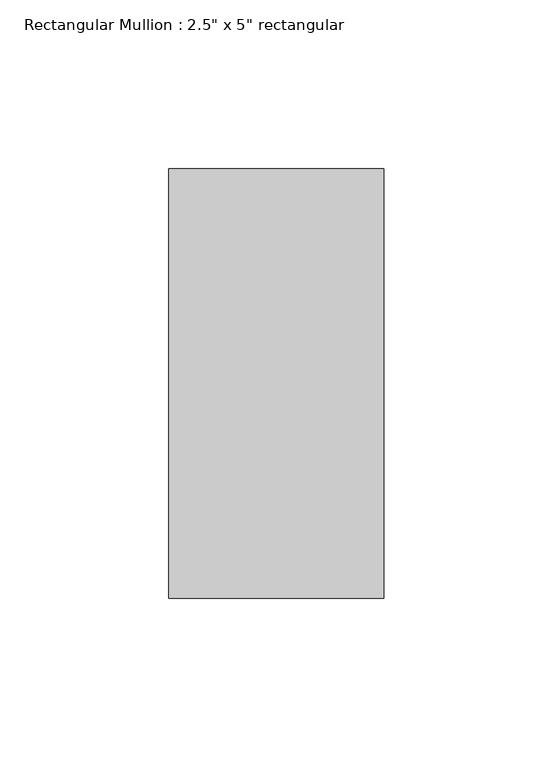
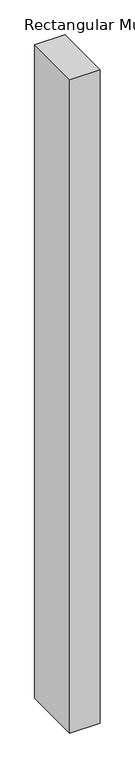
"""IFC4 building model written with IfcOpenShell, lengths in millimetres: member geometry."""

from ifc_helpers import new_model, si_unit, frame, origin, place, context, project, spatial, polyline, outline, extrude, source, transform, mapped, element, save


def member_b02ddeff(model_context):
    return source(origin(), model_context, "Body", "SweptSolid", [
        extrude(outline(polyline([(0.0, 63.5), (0.0, -63.5), (-63.5, -63.5), (-63.5, 63.5), (0.0, 63.5)])), frame((0.0, 0.0, -1446.9422272), z_axis=(0.0, 0.0, 1.0), x_axis=(1.0, 0.0, 0.0)), (0.0, 0.0, 1.0), 1446.9422272),
    ])


if __name__ == "__main__":
    model = new_model("IFC4")
    model_context = context("Model", 3, world=origin())
    ifc_project = project(units=[si_unit("LENGTHUNIT", "METRE", prefix="MILLI")], contexts=[model_context])
    site = spatial("IfcSite", under=ifc_project)
    building = spatial("IfcBuilding", under=site)
    placement = place(None, origin())
    member_shape = member_b02ddeff(model_context)
    element("IfcMember", 1, ObjectType="Rectangular Mullion : 2.5\" x 5\" rectangular", at=placement, inside=building, context=model_context, shape_type="MappedRepresentation", body=[
        mapped(member_shape, transform((0.0, 0.0, 0.0), x_axis=(1.0, 0.0, 0.0), y_axis=(0.0, 1.0, 0.0), z_axis=(0.0, 0.0, 1.0))),
    ])
    save(model, "model.ifc")

# Revit data of these elements
# Type "Rectangular Mullion : 2.5\" x 5\" rectangular"
#   built-in parameter 1007304 = 0.416667 (stored number, unit not read)
#   built-in parameter 1007301 = 0.104167 (stored number, unit not read)
#   built-in parameter 1007300 = 0.104167 (stored number, unit not read)
# Element 1 (IfcMember, "Rectangular Mullion : 2.5\" x 5\" rectangular")
#   Materials on its faces: "Aluminum"
# Materials
#   "Aluminum": class "Metal", colour RGB 247 247 247, transparency 0, Description = "Aluminum 6061", Cost = 0
